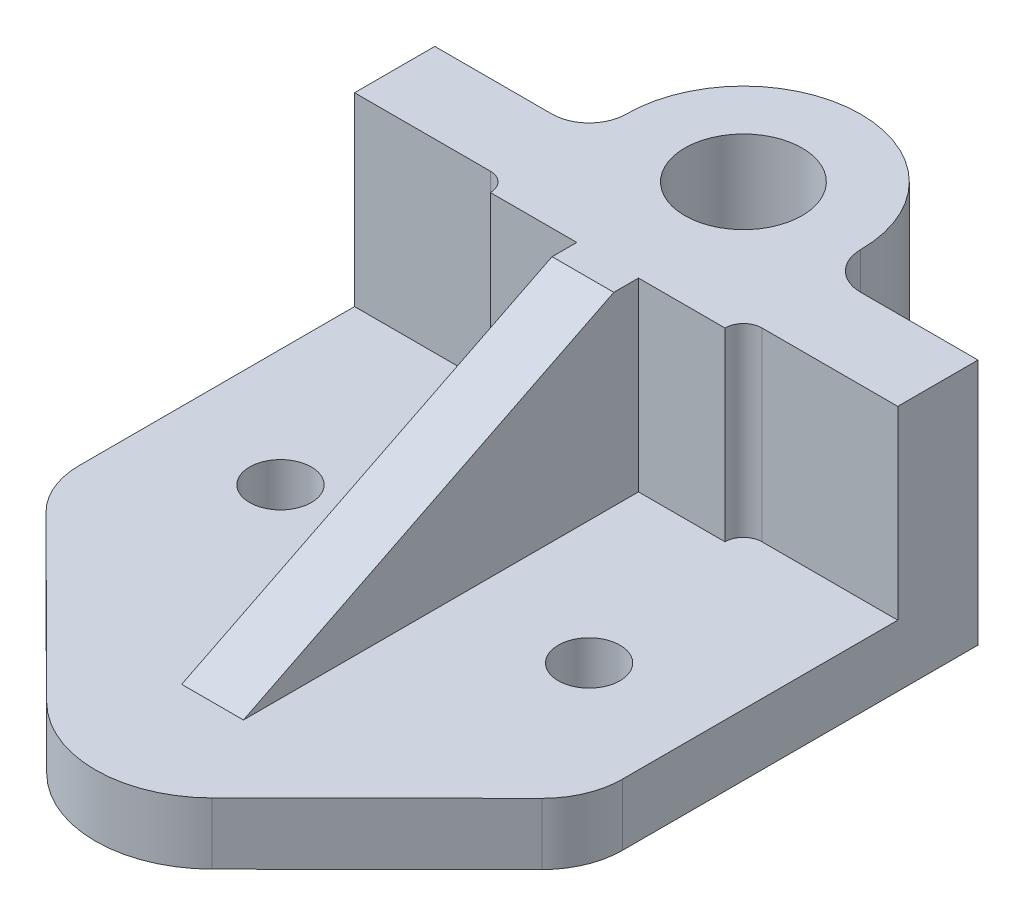
ISO-10303-21;
HEADER;
FILE_DESCRIPTION(('STEP AP214'),'2;1');
FILE_NAME('part.step','',(''),(''),'','','');
FILE_SCHEMA(('AUTOMOTIVE_DESIGN { 1 0 10303 214 1 1 1 1 }'));
ENDSEC;
DATA;
#1=APPLICATION_CONTEXT('core data for automotive mechanical design processes');
#2=APPLICATION_PROTOCOL_DEFINITION('international standard','automotive_design',2000,#1);
#3=PRODUCT_CONTEXT('',#1,'mechanical');
#4=PRODUCT('Part','Part','',(#3));
#5=PRODUCT_RELATED_PRODUCT_CATEGORY('part','',(#4));
#6=PRODUCT_DEFINITION_FORMATION('','',#4);
#7=PRODUCT_DEFINITION_CONTEXT('part definition',#1,'design');
#8=PRODUCT_DEFINITION('design','',#6,#7);
#9=PRODUCT_DEFINITION_SHAPE('','',#8);
#10=(LENGTH_UNIT() NAMED_UNIT(*) SI_UNIT(.MILLI.,.METRE.));
#11=(NAMED_UNIT(*) PLANE_ANGLE_UNIT() SI_UNIT($,.RADIAN.));
#12=(NAMED_UNIT(*) SI_UNIT($,.STERADIAN.) SOLID_ANGLE_UNIT());
#13=UNCERTAINTY_MEASURE_WITH_UNIT(LENGTH_MEASURE(1.E-05),#10,'distance_accuracy_value','');
#14=(GEOMETRIC_REPRESENTATION_CONTEXT(3) GLOBAL_UNCERTAINTY_ASSIGNED_CONTEXT((#13)) GLOBAL_UNIT_ASSIGNED_CONTEXT((#10,
#11,#12)) REPRESENTATION_CONTEXT('',''));
#15=CARTESIAN_POINT('',(0.,0.,0.));
#16=DIRECTION('',(0.,0.,1.));
#17=DIRECTION('',(1.,0.,0.));
#18=AXIS2_PLACEMENT_3D('',#15,#16,#17);
#19=CARTESIAN_POINT('',(-44.,40.,-6.5));
#20=DIRECTION('',(0.,0.,1.));
#21=DIRECTION('',(1.,0.,0.));
#22=AXIS2_PLACEMENT_3D('',#19,#20,#21);
#23=PLANE('',#22);
#24=DIRECTION('',(-1.,0.,0.));
#25=VECTOR('',#24,1.);
#26=CARTESIAN_POINT('',(-44.,0.,-6.5));
#27=LINE('',#26,#25);
#28=CARTESIAN_POINT('',(44.,0.,-6.5));
#29=VERTEX_POINT('',#28);
#30=CARTESIAN_POINT('',(25.,0.,-6.5));
#31=VERTEX_POINT('',#30);
#32=EDGE_CURVE('E291',#29,#31,#27,.T.);
#33=ORIENTED_EDGE('',*,*,#32,.T.);
#34=DIRECTION('',(0.,1.,0.));
#35=VECTOR('',#34,1.);
#36=CARTESIAN_POINT('',(25.,40.,-6.5));
#37=LINE('',#36,#35);
#38=CARTESIAN_POINT('',(25.,40.,-6.5));
#39=VERTEX_POINT('',#38);
#40=EDGE_CURVE('E339',#31,#39,#37,.T.);
#41=ORIENTED_EDGE('',*,*,#40,.T.);
#42=DIRECTION('',(-1.,0.,0.));
#43=VECTOR('',#42,1.);
#44=CARTESIAN_POINT('',(-44.,40.,-6.5));
#45=LINE('',#44,#43);
#46=CARTESIAN_POINT('',(44.,40.,-6.5));
#47=VERTEX_POINT('',#46);
#48=EDGE_CURVE('E281',#47,#39,#45,.T.);
#49=ORIENTED_EDGE('',*,*,#48,.F.);
#50=DIRECTION('',(0.,-1.,0.));
#51=VECTOR('',#50,1.);
#52=CARTESIAN_POINT('',(44.,40.,-6.5));
#53=LINE('',#52,#51);
#54=EDGE_CURVE('E306',#47,#29,#53,.T.);
#55=ORIENTED_EDGE('',*,*,#54,.T.);
#56=EDGE_LOOP('',(#33,#41,#49,#55));
#57=FACE_BOUND('',#56,.T.);
#58=ADVANCED_FACE('F44',(#57),#23,.F.);
#59=CARTESIAN_POINT('',(-44.,10.,56.5));
#60=DIRECTION('',(0.,-1.,0.));
#61=DIRECTION('',(1.,0.,0.));
#62=AXIS2_PLACEMENT_3D('',#59,#60,#61);
#63=PLANE('',#62);
#64=CARTESIAN_POINT('',(-25.,10.,37.5));
#65=DIRECTION('',(0.,1.,0.));
#66=DIRECTION('',(-1.,0.,0.));
#67=AXIS2_PLACEMENT_3D('',#64,#65,#66);
#68=CIRCLE('',#67,5.);
#69=CARTESIAN_POINT('',(-30.,10.,37.5));
#70=VERTEX_POINT('',#69);
#71=EDGE_CURVE('E382',#70,#70,#68,.T.);
#72=ORIENTED_EDGE('',*,*,#71,.F.);
#73=EDGE_LOOP('',(#72));
#74=FACE_BOUND('',#73,.T.);
#75=CARTESIAN_POINT('',(25.,10.,37.5));
#76=DIRECTION('',(0.,1.,0.));
#77=DIRECTION('',(-1.,0.,0.));
#78=AXIS2_PLACEMENT_3D('',#75,#76,#77);
#79=CIRCLE('',#78,5.);
#80=CARTESIAN_POINT('',(20.,10.,37.5));
#81=VERTEX_POINT('',#80);
#82=EDGE_CURVE('E222',#81,#81,#79,.T.);
#83=ORIENTED_EDGE('',*,*,#82,.F.);
#84=EDGE_LOOP('',(#83));
#85=FACE_BOUND('',#84,.T.);
#86=DIRECTION('',(0.,0.,-1.));
#87=VECTOR('',#86,1.);
#88=CARTESIAN_POINT('',(5.,10.,13.5));
#89=LINE('',#88,#87);
#90=CARTESIAN_POINT('',(5.,10.,73.5));
#91=VERTEX_POINT('',#90);
#92=CARTESIAN_POINT('',(5.,10.,9.5));
#93=VERTEX_POINT('',#92);
#94=EDGE_CURVE('E201',#91,#93,#89,.T.);
#95=ORIENTED_EDGE('',*,*,#94,.F.);
#96=DIRECTION('',(-1.,0.,0.));
#97=VECTOR('',#96,1.);
#98=CARTESIAN_POINT('',(-44.,10.,73.5));
#99=LINE('',#98,#97);
#100=CARTESIAN_POINT('',(-5.,10.,73.5));
#101=VERTEX_POINT('',#100);
#102=EDGE_CURVE('E219',#91,#101,#99,.T.);
#103=ORIENTED_EDGE('',*,*,#102,.T.);
#104=DIRECTION('',(0.,0.,-1.));
#105=VECTOR('',#104,1.);
#106=CARTESIAN_POINT('',(-5.,10.,13.5));
#107=LINE('',#106,#105);
#108=CARTESIAN_POINT('',(-5.,10.,9.5));
#109=VERTEX_POINT('',#108);
#110=EDGE_CURVE('E235',#101,#109,#107,.T.);
#111=ORIENTED_EDGE('',*,*,#110,.T.);
#112=DIRECTION('',(1.,0.,0.));
#113=VECTOR('',#112,1.);
#114=CARTESIAN_POINT('',(-19.,10.,9.5));
#115=LINE('',#114,#113);
#116=CARTESIAN_POINT('',(-19.,10.,9.5));
#117=VERTEX_POINT('',#116);
#118=EDGE_CURVE('E238',#117,#109,#115,.T.);
#119=ORIENTED_EDGE('',*,*,#118,.F.);
#120=CARTESIAN_POINT('',(-22.,10.,9.5));
#121=DIRECTION('',(0.,-1.,0.));
#122=DIRECTION('',(1.,0.,0.));
#123=AXIS2_PLACEMENT_3D('',#120,#121,#122);
#124=CIRCLE('',#123,3.);
#125=CARTESIAN_POINT('',(-22.,10.,6.5));
#126=VERTEX_POINT('',#125);
#127=EDGE_CURVE('E328',#117,#126,#124,.F.);
#128=ORIENTED_EDGE('',*,*,#127,.T.);
#129=DIRECTION('',(-1.,0.,0.));
#130=VECTOR('',#129,1.);
#131=CARTESIAN_POINT('',(-44.,10.,6.5));
#132=LINE('',#131,#130);
#133=CARTESIAN_POINT('',(-44.,10.,6.5));
#134=VERTEX_POINT('',#133);
#135=EDGE_CURVE('E262',#126,#134,#132,.T.);
#136=ORIENTED_EDGE('',*,*,#135,.T.);
#137=DIRECTION('',(0.,0.,-1.));
#138=VECTOR('',#137,1.);
#139=CARTESIAN_POINT('',(-44.,10.,56.5));
#140=LINE('',#139,#138);
#141=CARTESIAN_POINT('',(-44.,10.,51.0990021941588));
#142=VERTEX_POINT('',#141);
#143=EDGE_CURVE('E272',#142,#134,#140,.T.);
#144=ORIENTED_EDGE('',*,*,#143,.F.);
#145=CARTESIAN_POINT('',(-31.,10.,51.0990021941588));
#146=DIRECTION('',(0.,-1.,0.));
#147=DIRECTION('',(1.,0.,0.));
#148=AXIS2_PLACEMENT_3D('',#145,#146,#147);
#149=CIRCLE('',#148,13.);
#150=CARTESIAN_POINT('',(-40.1727948989015,10.,60.3109419324922));
#151=VERTEX_POINT('',#150);
#152=EDGE_CURVE('E315',#142,#151,#149,.F.);
#153=ORIENTED_EDGE('',*,*,#152,.T.);
#154=DIRECTION('',(0.708610749102569,0.,0.705599607607811));
#155=VECTOR('',#154,1.);
#156=CARTESIAN_POINT('',(-44.,10.,56.5));
#157=LINE('',#156,#155);
#158=CARTESIAN_POINT('',(-13.4063925445484,10.,86.9636042329488));
#159=VERTEX_POINT('',#158);
#160=EDGE_CURVE('E250',#151,#159,#157,.T.);
#161=ORIENTED_EDGE('',*,*,#160,.T.);
#162=CARTESIAN_POINT('',(0.,10.,73.5));
#163=DIRECTION('',(0.,1.,0.));
#164=DIRECTION('',(-1.,0.,0.));
#165=AXIS2_PLACEMENT_3D('',#162,#163,#164);
#166=CIRCLE('',#165,19.);
#167=CARTESIAN_POINT('',(13.4063925445484,10.,86.9636042329488));
#168=VERTEX_POINT('',#167);
#169=EDGE_CURVE('E259',#159,#168,#166,.T.);
#170=ORIENTED_EDGE('',*,*,#169,.T.);
#171=DIRECTION('',(0.708610749102569,0.,-0.705599607607811));
#172=VECTOR('',#171,1.);
#173=CARTESIAN_POINT('',(44.,10.,56.5));
#174=LINE('',#173,#172);
#175=CARTESIAN_POINT('',(40.1727948989016,10.,60.3109419324922));
#176=VERTEX_POINT('',#175);
#177=EDGE_CURVE('E252',#168,#176,#174,.T.);
#178=ORIENTED_EDGE('',*,*,#177,.T.);
#179=CARTESIAN_POINT('',(31.,10.,51.0990021941588));
#180=DIRECTION('',(0.,-1.,0.));
#181=DIRECTION('',(1.,0.,0.));
#182=AXIS2_PLACEMENT_3D('',#179,#180,#181);
#183=CIRCLE('',#182,13.);
#184=CARTESIAN_POINT('',(44.,10.,51.0990021941588));
#185=VERTEX_POINT('',#184);
#186=EDGE_CURVE('E313',#176,#185,#183,.F.);
#187=ORIENTED_EDGE('',*,*,#186,.T.);
#188=DIRECTION('',(0.,0.,-1.));
#189=VECTOR('',#188,1.);
#190=CARTESIAN_POINT('',(44.,10.,56.5));
#191=LINE('',#190,#189);
#192=CARTESIAN_POINT('',(44.,10.,6.5));
#193=VERTEX_POINT('',#192);
#194=EDGE_CURVE('E274',#185,#193,#191,.T.);
#195=ORIENTED_EDGE('',*,*,#194,.T.);
#196=CARTESIAN_POINT('',(22.,10.,6.5));
#197=VERTEX_POINT('',#196);
#198=EDGE_CURVE('E268',#193,#197,#132,.T.);
#199=ORIENTED_EDGE('',*,*,#198,.T.);
#200=CARTESIAN_POINT('',(22.,10.,9.5));
#201=DIRECTION('',(0.,-1.,0.));
#202=DIRECTION('',(1.,0.,0.));
#203=AXIS2_PLACEMENT_3D('',#200,#201,#202);
#204=CIRCLE('',#203,3.);
#205=CARTESIAN_POINT('',(19.,10.,9.5));
#206=VERTEX_POINT('',#205);
#207=EDGE_CURVE('E331',#197,#206,#204,.F.);
#208=ORIENTED_EDGE('',*,*,#207,.T.);
#209=EDGE_CURVE('E240',#93,#206,#115,.T.);
#210=ORIENTED_EDGE('',*,*,#209,.F.);
#211=EDGE_LOOP('',(#95,#103,#111,#119,#128,#136,#144,#153,#161,#170,#178,#187,#195,#199,#208,#210));
#212=FACE_BOUND('',#211,.T.);
#213=ADVANCED_FACE('F391',(#74,#85,#212),#63,.F.);
#214=CARTESIAN_POINT('',(0.,0.,9.5));
#215=DIRECTION('',(0.,0.,1.));
#216=DIRECTION('',(1.,0.,0.));
#217=AXIS2_PLACEMENT_3D('',#214,#215,#216);
#218=PLANE('',#217);
#219=ORIENTED_EDGE('',*,*,#118,.T.);
#220=DIRECTION('',(0.,-1.,0.));
#221=VECTOR('',#220,1.);
#222=CARTESIAN_POINT('',(-5.,40.,9.5));
#223=LINE('',#222,#221);
#224=CARTESIAN_POINT('',(-5.,40.,9.5));
#225=VERTEX_POINT('',#224);
#226=EDGE_CURVE('E218',#225,#109,#223,.T.);
#227=ORIENTED_EDGE('',*,*,#226,.F.);
#228=DIRECTION('',(-1.,0.,0.));
#229=VECTOR('',#228,1.);
#230=CARTESIAN_POINT('',(-19.,40.,9.5));
#231=LINE('',#230,#229);
#232=CARTESIAN_POINT('',(-19.,40.,9.5));
#233=VERTEX_POINT('',#232);
#234=EDGE_CURVE('E242',#225,#233,#231,.T.);
#235=ORIENTED_EDGE('',*,*,#234,.T.);
#236=DIRECTION('',(0.,-1.,0.));
#237=VECTOR('',#236,1.);
#238=CARTESIAN_POINT('',(-19.,40.,9.5));
#239=LINE('',#238,#237);
#240=EDGE_CURVE('E234',#233,#117,#239,.T.);
#241=ORIENTED_EDGE('',*,*,#240,.T.);
#242=EDGE_LOOP('',(#219,#227,#235,#241));
#243=FACE_BOUND('',#242,.T.);
#244=ADVANCED_FACE('F392',(#243),#218,.T.);
#245=CARTESIAN_POINT('',(19.,40.,9.5));
#246=VERTEX_POINT('',#245);
#247=CARTESIAN_POINT('',(4.99999999999999,40.,9.5));
#248=VERTEX_POINT('',#247);
#249=EDGE_CURVE('E244',#246,#248,#231,.T.);
#250=ORIENTED_EDGE('',*,*,#249,.T.);
#251=DIRECTION('',(0.,1.,0.));
#252=VECTOR('',#251,1.);
#253=CARTESIAN_POINT('',(5.,40.,9.5));
#254=LINE('',#253,#252);
#255=EDGE_CURVE('E198',#93,#248,#254,.T.);
#256=ORIENTED_EDGE('',*,*,#255,.F.);
#257=ORIENTED_EDGE('',*,*,#209,.T.);
#258=DIRECTION('',(0.,1.,0.));
#259=VECTOR('',#258,1.);
#260=CARTESIAN_POINT('',(19.,40.,9.5));
#261=LINE('',#260,#259);
#262=EDGE_CURVE('E241',#206,#246,#261,.T.);
#263=ORIENTED_EDGE('',*,*,#262,.T.);
#264=EDGE_LOOP('',(#250,#256,#257,#263));
#265=FACE_BOUND('',#264,.T.);
#266=ADVANCED_FACE('F401',(#265),#218,.T.);
#267=CARTESIAN_POINT('',(-44.,40.,6.5));
#268=DIRECTION('',(0.,0.,-1.));
#269=DIRECTION('',(-1.,0.,0.));
#270=AXIS2_PLACEMENT_3D('',#267,#268,#269);
#271=PLANE('',#270);
#272=ORIENTED_EDGE('',*,*,#135,.F.);
#273=DIRECTION('',(0.,-1.,0.));
#274=VECTOR('',#273,1.);
#275=CARTESIAN_POINT('',(-22.,40.,6.5));
#276=LINE('',#275,#274);
#277=CARTESIAN_POINT('',(-22.,40.,6.5));
#278=VERTEX_POINT('',#277);
#279=EDGE_CURVE('E333',#126,#278,#276,.F.);
#280=ORIENTED_EDGE('',*,*,#279,.T.);
#281=DIRECTION('',(1.,0.,0.));
#282=VECTOR('',#281,1.);
#283=CARTESIAN_POINT('',(-44.,40.,6.5));
#284=LINE('',#283,#282);
#285=CARTESIAN_POINT('',(-44.,40.,6.5));
#286=VERTEX_POINT('',#285);
#287=EDGE_CURVE('E290',#286,#278,#284,.T.);
#288=ORIENTED_EDGE('',*,*,#287,.F.);
#289=DIRECTION('',(0.,-1.,0.));
#290=VECTOR('',#289,1.);
#291=CARTESIAN_POINT('',(-44.,40.,6.5));
#292=LINE('',#291,#290);
#293=EDGE_CURVE('E297',#286,#134,#292,.T.);
#294=ORIENTED_EDGE('',*,*,#293,.T.);
#295=EDGE_LOOP('',(#272,#280,#288,#294));
#296=FACE_BOUND('',#295,.T.);
#297=ADVANCED_FACE('F449',(#296),#271,.F.);
#298=CARTESIAN_POINT('',(22.,40.,6.5));
#299=VERTEX_POINT('',#298);
#300=CARTESIAN_POINT('',(44.,40.,6.5));
#301=VERTEX_POINT('',#300);
#302=EDGE_CURVE('E286',#299,#301,#284,.T.);
#303=ORIENTED_EDGE('',*,*,#302,.F.);
#304=DIRECTION('',(0.,1.,0.));
#305=VECTOR('',#304,1.);
#306=CARTESIAN_POINT('',(22.,10.,6.5));
#307=LINE('',#306,#305);
#308=EDGE_CURVE('E326',#299,#197,#307,.F.);
#309=ORIENTED_EDGE('',*,*,#308,.T.);
#310=ORIENTED_EDGE('',*,*,#198,.F.);
#311=DIRECTION('',(0.,-1.,0.));
#312=VECTOR('',#311,1.);
#313=CARTESIAN_POINT('',(44.,40.,6.5));
#314=LINE('',#313,#312);
#315=EDGE_CURVE('E289',#301,#193,#314,.T.);
#316=ORIENTED_EDGE('',*,*,#315,.F.);
#317=EDGE_LOOP('',(#303,#309,#310,#316));
#318=FACE_BOUND('',#317,.T.);
#319=ADVANCED_FACE('F408',(#318),#271,.F.);
#320=CARTESIAN_POINT('',(44.,40.,6.5));
#321=DIRECTION('',(-1.,0.,0.));
#322=DIRECTION('',(0.,0.,1.));
#323=AXIS2_PLACEMENT_3D('',#320,#321,#322);
#324=PLANE('',#323);
#325=ORIENTED_EDGE('',*,*,#194,.F.);
#326=DIRECTION('',(0.,1.,0.));
#327=VECTOR('',#326,1.);
#328=CARTESIAN_POINT('',(44.,0.,51.0990021941588));
#329=LINE('',#328,#327);
#330=CARTESIAN_POINT('',(44.,0.,51.0990021941588));
#331=VERTEX_POINT('',#330);
#332=EDGE_CURVE('E317',#185,#331,#329,.F.);
#333=ORIENTED_EDGE('',*,*,#332,.T.);
#334=DIRECTION('',(0.,0.,-1.));
#335=VECTOR('',#334,1.);
#336=CARTESIAN_POINT('',(44.,0.,6.5));
#337=LINE('',#336,#335);
#338=EDGE_CURVE('E277',#331,#29,#337,.T.);
#339=ORIENTED_EDGE('',*,*,#338,.T.);
#340=ORIENTED_EDGE('',*,*,#54,.F.);
#341=DIRECTION('',(0.,0.,-1.));
#342=VECTOR('',#341,1.);
#343=CARTESIAN_POINT('',(44.,40.,6.5));
#344=LINE('',#343,#342);
#345=EDGE_CURVE('E280',#301,#47,#344,.T.);
#346=ORIENTED_EDGE('',*,*,#345,.F.);
#347=ORIENTED_EDGE('',*,*,#315,.T.);
#348=EDGE_LOOP('',(#325,#333,#339,#340,#346,#347));
#349=FACE_BOUND('',#348,.T.);
#350=ADVANCED_FACE('F412',(#349),#324,.F.);
#351=CARTESIAN_POINT('',(-25.,40.,-6.5));
#352=VERTEX_POINT('',#351);
#353=CARTESIAN_POINT('',(-44.,40.,-6.5));
#354=VERTEX_POINT('',#353);
#355=EDGE_CURVE('E278',#352,#354,#45,.T.);
#356=ORIENTED_EDGE('',*,*,#355,.F.);
#357=DIRECTION('',(0.,1.,0.));
#358=VECTOR('',#357,1.);
#359=CARTESIAN_POINT('',(-25.,40.,-6.5));
#360=LINE('',#359,#358);
#361=CARTESIAN_POINT('',(-25.,0.,-6.5));
#362=VERTEX_POINT('',#361);
#363=EDGE_CURVE('E58',#352,#362,#360,.F.);
#364=ORIENTED_EDGE('',*,*,#363,.T.);
#365=CARTESIAN_POINT('',(-44.,0.,-6.5));
#366=VERTEX_POINT('',#365);
#367=EDGE_CURVE('E292',#362,#366,#27,.T.);
#368=ORIENTED_EDGE('',*,*,#367,.T.);
#369=DIRECTION('',(0.,-1.,0.));
#370=VECTOR('',#369,1.);
#371=CARTESIAN_POINT('',(-44.,40.,-6.5));
#372=LINE('',#371,#370);
#373=EDGE_CURVE('E303',#354,#366,#372,.T.);
#374=ORIENTED_EDGE('',*,*,#373,.F.);
#375=EDGE_LOOP('',(#356,#364,#368,#374));
#376=FACE_BOUND('',#375,.T.);
#377=ADVANCED_FACE('F472',(#376),#23,.F.);
#378=CARTESIAN_POINT('',(-44.,40.,6.5));
#379=DIRECTION('',(1.,0.,0.));
#380=DIRECTION('',(0.,0.,-1.));
#381=AXIS2_PLACEMENT_3D('',#378,#379,#380);
#382=PLANE('',#381);
#383=DIRECTION('',(0.,0.,1.));
#384=VECTOR('',#383,1.);
#385=CARTESIAN_POINT('',(-44.,0.,6.5));
#386=LINE('',#385,#384);
#387=CARTESIAN_POINT('',(-44.,0.,51.0990021941588));
#388=VERTEX_POINT('',#387);
#389=EDGE_CURVE('E284',#366,#388,#386,.T.);
#390=ORIENTED_EDGE('',*,*,#389,.T.);
#391=DIRECTION('',(0.,-1.,0.));
#392=VECTOR('',#391,1.);
#393=CARTESIAN_POINT('',(-44.,10.,51.0990021941588));
#394=LINE('',#393,#392);
#395=EDGE_CURVE('E323',#388,#142,#394,.F.);
#396=ORIENTED_EDGE('',*,*,#395,.T.);
#397=ORIENTED_EDGE('',*,*,#143,.T.);
#398=ORIENTED_EDGE('',*,*,#293,.F.);
#399=DIRECTION('',(0.,0.,1.));
#400=VECTOR('',#399,1.);
#401=CARTESIAN_POINT('',(-44.,40.,6.5));
#402=LINE('',#401,#400);
#403=EDGE_CURVE('E283',#354,#286,#402,.T.);
#404=ORIENTED_EDGE('',*,*,#403,.F.);
#405=ORIENTED_EDGE('',*,*,#373,.T.);
#406=EDGE_LOOP('',(#390,#396,#397,#398,#404,#405));
#407=FACE_BOUND('',#406,.T.);
#408=ADVANCED_FACE('F445',(#407),#382,.F.);
#409=CARTESIAN_POINT('',(0.,40.,0.));
#410=DIRECTION('',(0.,-1.,0.));
#411=DIRECTION('',(0.,0.,-1.));
#412=AXIS2_PLACEMENT_3D('',#409,#410,#411);
#413=PLANE('',#412);
#414=CARTESIAN_POINT('',(0.,40.,-12.5));
#415=DIRECTION('',(0.,1.,0.));
#416=DIRECTION('',(0.,0.,1.));
#417=AXIS2_PLACEMENT_3D('',#414,#415,#416);
#418=CIRCLE('',#417,9.5);
#419=CARTESIAN_POINT('',(0.,40.,-3.));
#420=VERTEX_POINT('',#419);
#421=EDGE_CURVE('E374',#420,#420,#418,.T.);
#422=ORIENTED_EDGE('',*,*,#421,.F.);
#423=EDGE_LOOP('',(#422));
#424=FACE_BOUND('',#423,.T.);
#425=ORIENTED_EDGE('',*,*,#48,.T.);
#426=CARTESIAN_POINT('',(25.,40.,-12.5));
#427=DIRECTION('',(0.,-1.,0.));
#428=DIRECTION('',(0.,0.,-1.));
#429=AXIS2_PLACEMENT_3D('',#426,#427,#428);
#430=CIRCLE('',#429,6.);
#431=CARTESIAN_POINT('',(19.,40.,-12.5));
#432=VERTEX_POINT('',#431);
#433=EDGE_CURVE('E350',#39,#432,#430,.T.);
#434=ORIENTED_EDGE('',*,*,#433,.T.);
#435=CARTESIAN_POINT('',(0.,40.,-12.5));
#436=DIRECTION('',(0.,1.,0.));
#437=DIRECTION('',(0.,0.,1.));
#438=AXIS2_PLACEMENT_3D('',#435,#436,#437);
#439=CIRCLE('',#438,19.);
#440=CARTESIAN_POINT('',(-19.,40.,-12.5));
#441=VERTEX_POINT('',#440);
#442=EDGE_CURVE('E370',#432,#441,#439,.T.);
#443=ORIENTED_EDGE('',*,*,#442,.T.);
#444=CARTESIAN_POINT('',(-25.,40.,-12.5));
#445=DIRECTION('',(0.,-1.,0.));
#446=DIRECTION('',(0.,0.,-1.));
#447=AXIS2_PLACEMENT_3D('',#444,#445,#446);
#448=CIRCLE('',#447,6.);
#449=EDGE_CURVE('E52',#441,#352,#448,.T.);
#450=ORIENTED_EDGE('',*,*,#449,.T.);
#451=ORIENTED_EDGE('',*,*,#355,.T.);
#452=ORIENTED_EDGE('',*,*,#403,.T.);
#453=ORIENTED_EDGE('',*,*,#287,.T.);
#454=CARTESIAN_POINT('',(-22.,40.,9.5));
#455=DIRECTION('',(0.,-1.,0.));
#456=DIRECTION('',(0.,0.,-1.));
#457=AXIS2_PLACEMENT_3D('',#454,#455,#456);
#458=CIRCLE('',#457,3.);
#459=EDGE_CURVE('E340',#278,#233,#458,.T.);
#460=ORIENTED_EDGE('',*,*,#459,.T.);
#461=ORIENTED_EDGE('',*,*,#234,.F.);
#462=DIRECTION('',(0.,0.,-1.));
#463=VECTOR('',#462,1.);
#464=CARTESIAN_POINT('',(-5.,40.,13.5));
#465=LINE('',#464,#463);
#466=CARTESIAN_POINT('',(-5.,40.,13.5));
#467=VERTEX_POINT('',#466);
#468=EDGE_CURVE('E205',#467,#225,#465,.T.);
#469=ORIENTED_EDGE('',*,*,#468,.F.);
#470=DIRECTION('',(-1.,0.,0.));
#471=VECTOR('',#470,1.);
#472=CARTESIAN_POINT('',(-5.,40.,13.5));
#473=LINE('',#472,#471);
#474=CARTESIAN_POINT('',(5.,40.,13.5));
#475=VERTEX_POINT('',#474);
#476=EDGE_CURVE('E204',#475,#467,#473,.T.);
#477=ORIENTED_EDGE('',*,*,#476,.F.);
#478=DIRECTION('',(0.,0.,-1.));
#479=VECTOR('',#478,1.);
#480=CARTESIAN_POINT('',(5.,40.,13.5));
#481=LINE('',#480,#479);
#482=EDGE_CURVE('E194',#475,#248,#481,.T.);
#483=ORIENTED_EDGE('',*,*,#482,.T.);
#484=ORIENTED_EDGE('',*,*,#249,.F.);
#485=CARTESIAN_POINT('',(22.,40.,9.5));
#486=DIRECTION('',(0.,-1.,0.));
#487=DIRECTION('',(0.,0.,-1.));
#488=AXIS2_PLACEMENT_3D('',#485,#486,#487);
#489=CIRCLE('',#488,3.);
#490=EDGE_CURVE('E334',#246,#299,#489,.T.);
#491=ORIENTED_EDGE('',*,*,#490,.T.);
#492=ORIENTED_EDGE('',*,*,#302,.T.);
#493=ORIENTED_EDGE('',*,*,#345,.T.);
#494=EDGE_LOOP('',(#425,#434,#443,#450,#451,#452,#453,#460,#461,#469,#477,#483,#484,#491,#492,#493));
#495=FACE_BOUND('',#494,.T.);
#496=ADVANCED_FACE('F210',(#424,#495),#413,.F.);
#497=CARTESIAN_POINT('',(0.,0.,0.));
#498=DIRECTION('',(0.,-1.,0.));
#499=DIRECTION('',(0.,0.,-1.));
#500=AXIS2_PLACEMENT_3D('',#497,#498,#499);
#501=PLANE('',#500);
#502=CARTESIAN_POINT('',(0.,0.,-12.5));
#503=DIRECTION('',(0.,1.,0.));
#504=DIRECTION('',(0.,0.,1.));
#505=AXIS2_PLACEMENT_3D('',#502,#503,#504);
#506=CIRCLE('',#505,9.5);
#507=CARTESIAN_POINT('',(0.,0.,-3.));
#508=VERTEX_POINT('',#507);
#509=EDGE_CURVE('E371',#508,#508,#506,.T.);
#510=ORIENTED_EDGE('',*,*,#509,.T.);
#511=EDGE_LOOP('',(#510));
#512=FACE_BOUND('',#511,.T.);
#513=CARTESIAN_POINT('',(-25.,0.,37.5));
#514=DIRECTION('',(0.,1.,0.));
#515=DIRECTION('',(-1.,0.,0.));
#516=AXIS2_PLACEMENT_3D('',#513,#514,#515);
#517=CIRCLE('',#516,5.);
#518=CARTESIAN_POINT('',(-30.,0.,37.5));
#519=VERTEX_POINT('',#518);
#520=EDGE_CURVE('E221',#519,#519,#517,.T.);
#521=ORIENTED_EDGE('',*,*,#520,.T.);
#522=EDGE_LOOP('',(#521));
#523=FACE_BOUND('',#522,.T.);
#524=CARTESIAN_POINT('',(25.,0.,37.5));
#525=DIRECTION('',(0.,1.,0.));
#526=DIRECTION('',(-1.,0.,0.));
#527=AXIS2_PLACEMENT_3D('',#524,#525,#526);
#528=CIRCLE('',#527,5.);
#529=CARTESIAN_POINT('',(20.,0.,37.5));
#530=VERTEX_POINT('',#529);
#531=EDGE_CURVE('E384',#530,#530,#528,.T.);
#532=ORIENTED_EDGE('',*,*,#531,.T.);
#533=EDGE_LOOP('',(#532));
#534=FACE_BOUND('',#533,.T.);
#535=DIRECTION('',(0.708610749102569,0.,-0.705599607607811));
#536=VECTOR('',#535,1.);
#537=CARTESIAN_POINT('',(44.,0.,56.5));
#538=LINE('',#537,#536);
#539=CARTESIAN_POINT('',(13.4063925445484,0.,86.9636042329488));
#540=VERTEX_POINT('',#539);
#541=CARTESIAN_POINT('',(40.1727948989016,0.,60.3109419324922));
#542=VERTEX_POINT('',#541);
#543=EDGE_CURVE('E254',#540,#542,#538,.T.);
#544=ORIENTED_EDGE('',*,*,#543,.F.);
#545=CARTESIAN_POINT('',(0.,0.,73.5));
#546=DIRECTION('',(0.,1.,0.));
#547=DIRECTION('',(-1.,0.,0.));
#548=AXIS2_PLACEMENT_3D('',#545,#546,#547);
#549=CIRCLE('',#548,19.);
#550=CARTESIAN_POINT('',(-13.4063925445484,0.,86.9636042329488));
#551=VERTEX_POINT('',#550);
#552=EDGE_CURVE('E249',#551,#540,#549,.T.);
#553=ORIENTED_EDGE('',*,*,#552,.F.);
#554=DIRECTION('',(0.708610749102569,0.,0.705599607607811));
#555=VECTOR('',#554,1.);
#556=CARTESIAN_POINT('',(-44.,0.,56.5));
#557=LINE('',#556,#555);
#558=CARTESIAN_POINT('',(-40.1727948989015,0.,60.3109419324922));
#559=VERTEX_POINT('',#558);
#560=EDGE_CURVE('E247',#559,#551,#557,.T.);
#561=ORIENTED_EDGE('',*,*,#560,.F.);
#562=CARTESIAN_POINT('',(-31.,0.,51.0990021941588));
#563=DIRECTION('',(0.,-1.,0.));
#564=DIRECTION('',(0.,0.,-1.));
#565=AXIS2_PLACEMENT_3D('',#562,#563,#564);
#566=CIRCLE('',#565,13.);
#567=EDGE_CURVE('E319',#559,#388,#566,.T.);
#568=ORIENTED_EDGE('',*,*,#567,.T.);
#569=ORIENTED_EDGE('',*,*,#389,.F.);
#570=ORIENTED_EDGE('',*,*,#367,.F.);
#571=CARTESIAN_POINT('',(-25.,0.,-12.5));
#572=DIRECTION('',(0.,-1.,0.));
#573=DIRECTION('',(0.,0.,-1.));
#574=AXIS2_PLACEMENT_3D('',#571,#572,#573);
#575=CIRCLE('',#574,6.);
#576=CARTESIAN_POINT('',(-19.,0.,-12.5));
#577=VERTEX_POINT('',#576);
#578=EDGE_CURVE('E11',#362,#577,#575,.F.);
#579=ORIENTED_EDGE('',*,*,#578,.T.);
#580=CARTESIAN_POINT('',(0.,0.,-12.5));
#581=DIRECTION('',(0.,1.,0.));
#582=DIRECTION('',(0.,0.,1.));
#583=AXIS2_PLACEMENT_3D('',#580,#581,#582);
#584=CIRCLE('',#583,19.);
#585=CARTESIAN_POINT('',(19.,0.,-12.5));
#586=VERTEX_POINT('',#585);
#587=EDGE_CURVE('E360',#586,#577,#584,.T.);
#588=ORIENTED_EDGE('',*,*,#587,.F.);
#589=CARTESIAN_POINT('',(25.,0.,-12.5));
#590=DIRECTION('',(0.,-1.,0.));
#591=DIRECTION('',(0.,0.,-1.));
#592=AXIS2_PLACEMENT_3D('',#589,#590,#591);
#593=CIRCLE('',#592,6.);
#594=EDGE_CURVE('E347',#586,#31,#593,.F.);
#595=ORIENTED_EDGE('',*,*,#594,.T.);
#596=ORIENTED_EDGE('',*,*,#32,.F.);
#597=ORIENTED_EDGE('',*,*,#338,.F.);
#598=CARTESIAN_POINT('',(31.,0.,51.0990021941588));
#599=DIRECTION('',(0.,-1.,0.));
#600=DIRECTION('',(0.,0.,-1.));
#601=AXIS2_PLACEMENT_3D('',#598,#599,#600);
#602=CIRCLE('',#601,13.);
#603=EDGE_CURVE('E318',#331,#542,#602,.T.);
#604=ORIENTED_EDGE('',*,*,#603,.T.);
#605=EDGE_LOOP('',(#544,#553,#561,#568,#569,#570,#579,#588,#595,#596,#597,#604));
#606=FACE_BOUND('',#605,.T.);
#607=ADVANCED_FACE('F358',(#512,#523,#534,#606),#501,.T.);
#608=CARTESIAN_POINT('',(44.,0.,56.5));
#609=DIRECTION('',(0.705599607607811,0.,0.708610749102569));
#610=DIRECTION('',(0.708610749102569,0.,-0.705599607607811));
#611=AXIS2_PLACEMENT_3D('',#608,#609,#610);
#612=PLANE('',#611);
#613=ORIENTED_EDGE('',*,*,#543,.T.);
#614=DIRECTION('',(0.,1.,0.));
#615=VECTOR('',#614,1.);
#616=CARTESIAN_POINT('',(40.1727948989016,10.,60.3109419324922));
#617=LINE('',#616,#615);
#618=EDGE_CURVE('E307',#542,#176,#617,.T.);
#619=ORIENTED_EDGE('',*,*,#618,.T.);
#620=ORIENTED_EDGE('',*,*,#177,.F.);
#621=DIRECTION('',(0.,1.,0.));
#622=VECTOR('',#621,1.);
#623=CARTESIAN_POINT('',(13.4063925445484,0.,86.9636042329488));
#624=LINE('',#623,#622);
#625=EDGE_CURVE('E265',#540,#168,#624,.T.);
#626=ORIENTED_EDGE('',*,*,#625,.F.);
#627=EDGE_LOOP('',(#613,#619,#620,#626));
#628=FACE_BOUND('',#627,.T.);
#629=ADVANCED_FACE('F421',(#628),#612,.T.);
#630=CARTESIAN_POINT('',(0.,0.,73.5));
#631=DIRECTION('',(0.,1.,0.));
#632=DIRECTION('',(-1.,0.,0.));
#633=AXIS2_PLACEMENT_3D('',#630,#631,#632);
#634=CYLINDRICAL_SURFACE('',#633,19.);
#635=ORIENTED_EDGE('',*,*,#552,.T.);
#636=ORIENTED_EDGE('',*,*,#625,.T.);
#637=ORIENTED_EDGE('',*,*,#169,.F.);
#638=DIRECTION('',(0.,1.,0.));
#639=VECTOR('',#638,1.);
#640=CARTESIAN_POINT('',(-13.4063925445484,0.,86.9636042329488));
#641=LINE('',#640,#639);
#642=EDGE_CURVE('E257',#551,#159,#641,.T.);
#643=ORIENTED_EDGE('',*,*,#642,.F.);
#644=EDGE_LOOP('',(#635,#636,#637,#643));
#645=FACE_BOUND('',#644,.T.);
#646=ADVANCED_FACE('F429',(#645),#634,.T.);
#647=CARTESIAN_POINT('',(-44.,0.,56.5));
#648=DIRECTION('',(-0.705599607607811,0.,0.708610749102569));
#649=DIRECTION('',(0.708610749102569,0.,0.705599607607811));
#650=AXIS2_PLACEMENT_3D('',#647,#648,#649);
#651=PLANE('',#650);
#652=ORIENTED_EDGE('',*,*,#160,.F.);
#653=DIRECTION('',(0.,-1.,0.));
#654=VECTOR('',#653,1.);
#655=CARTESIAN_POINT('',(-40.1727948989015,0.,60.3109419324922));
#656=LINE('',#655,#654);
#657=EDGE_CURVE('E325',#151,#559,#656,.T.);
#658=ORIENTED_EDGE('',*,*,#657,.T.);
#659=ORIENTED_EDGE('',*,*,#560,.T.);
#660=ORIENTED_EDGE('',*,*,#642,.T.);
#661=EDGE_LOOP('',(#652,#658,#659,#660));
#662=FACE_BOUND('',#661,.T.);
#663=ADVANCED_FACE('F432',(#662),#651,.T.);
#664=CARTESIAN_POINT('',(31.,0.,51.0990021941588));
#665=DIRECTION('',(0.,-1.,0.));
#666=DIRECTION('',(0.,0.,-1.));
#667=AXIS2_PLACEMENT_3D('',#664,#665,#666);
#668=CYLINDRICAL_SURFACE('',#667,13.);
#669=ORIENTED_EDGE('',*,*,#603,.F.);
#670=ORIENTED_EDGE('',*,*,#332,.F.);
#671=ORIENTED_EDGE('',*,*,#186,.F.);
#672=ORIENTED_EDGE('',*,*,#618,.F.);
#673=EDGE_LOOP('',(#669,#670,#671,#672));
#674=FACE_BOUND('',#673,.T.);
#675=ADVANCED_FACE('F419',(#674),#668,.T.);
#676=CARTESIAN_POINT('',(-31.,0.,51.0990021941588));
#677=DIRECTION('',(0.,1.,0.));
#678=DIRECTION('',(0.,0.,1.));
#679=AXIS2_PLACEMENT_3D('',#676,#677,#678);
#680=CYLINDRICAL_SURFACE('',#679,13.);
#681=ORIENTED_EDGE('',*,*,#152,.F.);
#682=ORIENTED_EDGE('',*,*,#395,.F.);
#683=ORIENTED_EDGE('',*,*,#567,.F.);
#684=ORIENTED_EDGE('',*,*,#657,.F.);
#685=EDGE_LOOP('',(#681,#682,#683,#684));
#686=FACE_BOUND('',#685,.T.);
#687=ADVANCED_FACE('F438',(#686),#680,.T.);
#688=CARTESIAN_POINT('',(-5.,40.,13.5));
#689=DIRECTION('',(1.,0.,0.));
#690=DIRECTION('',(0.,1.,0.));
#691=AXIS2_PLACEMENT_3D('',#688,#689,#690);
#692=PLANE('',#691);
#693=ORIENTED_EDGE('',*,*,#226,.T.);
#694=ORIENTED_EDGE('',*,*,#110,.F.);
#695=DIRECTION('',(0.,-0.447213595499958,0.894427190999916));
#696=VECTOR('',#695,1.);
#697=CARTESIAN_POINT('',(-5.,40.,13.5));
#698=LINE('',#697,#696);
#699=EDGE_CURVE('E216',#467,#101,#698,.T.);
#700=ORIENTED_EDGE('',*,*,#699,.F.);
#701=ORIENTED_EDGE('',*,*,#468,.T.);
#702=EDGE_LOOP('',(#693,#694,#700,#701));
#703=FACE_BOUND('',#702,.T.);
#704=ADVANCED_FACE('F460',(#703),#692,.F.);
#705=CARTESIAN_POINT('',(5.,40.,13.5));
#706=DIRECTION('',(-1.,0.,0.));
#707=DIRECTION('',(0.,-1.,0.));
#708=AXIS2_PLACEMENT_3D('',#705,#706,#707);
#709=PLANE('',#708);
#710=ORIENTED_EDGE('',*,*,#255,.T.);
#711=ORIENTED_EDGE('',*,*,#482,.F.);
#712=DIRECTION('',(0.,-0.447213595499958,0.894427190999916));
#713=VECTOR('',#712,1.);
#714=CARTESIAN_POINT('',(5.,40.,13.5));
#715=LINE('',#714,#713);
#716=EDGE_CURVE('E200',#475,#91,#715,.T.);
#717=ORIENTED_EDGE('',*,*,#716,.T.);
#718=ORIENTED_EDGE('',*,*,#94,.T.);
#719=EDGE_LOOP('',(#710,#711,#717,#718));
#720=FACE_BOUND('',#719,.T.);
#721=ADVANCED_FACE('F193',(#720),#709,.F.);
#722=CARTESIAN_POINT('',(22.,40.,9.5));
#723=DIRECTION('',(0.,-1.,0.));
#724=DIRECTION('',(1.,0.,0.));
#725=AXIS2_PLACEMENT_3D('',#722,#723,#724);
#726=CYLINDRICAL_SURFACE('',#725,3.);
#727=ORIENTED_EDGE('',*,*,#207,.F.);
#728=ORIENTED_EDGE('',*,*,#308,.F.);
#729=ORIENTED_EDGE('',*,*,#490,.F.);
#730=ORIENTED_EDGE('',*,*,#262,.F.);
#731=EDGE_LOOP('',(#727,#728,#729,#730));
#732=FACE_BOUND('',#731,.T.);
#733=ADVANCED_FACE('F403',(#732),#726,.F.);
#734=CARTESIAN_POINT('',(-22.,40.,9.5));
#735=DIRECTION('',(0.,1.,0.));
#736=DIRECTION('',(-1.,0.,0.));
#737=AXIS2_PLACEMENT_3D('',#734,#735,#736);
#738=CYLINDRICAL_SURFACE('',#737,3.);
#739=ORIENTED_EDGE('',*,*,#459,.F.);
#740=ORIENTED_EDGE('',*,*,#279,.F.);
#741=ORIENTED_EDGE('',*,*,#127,.F.);
#742=ORIENTED_EDGE('',*,*,#240,.F.);
#743=EDGE_LOOP('',(#739,#740,#741,#742));
#744=FACE_BOUND('',#743,.T.);
#745=ADVANCED_FACE('F455',(#744),#738,.F.);
#746=CARTESIAN_POINT('',(0.,40.,13.5));
#747=DIRECTION('',(0.,0.894427190999916,0.447213595499958));
#748=DIRECTION('',(0.,-0.447213595499958,0.894427190999916));
#749=AXIS2_PLACEMENT_3D('',#746,#747,#748);
#750=PLANE('',#749);
#751=ORIENTED_EDGE('',*,*,#102,.F.);
#752=ORIENTED_EDGE('',*,*,#716,.F.);
#753=ORIENTED_EDGE('',*,*,#476,.T.);
#754=ORIENTED_EDGE('',*,*,#699,.T.);
#755=EDGE_LOOP('',(#751,#752,#753,#754));
#756=FACE_BOUND('',#755,.T.);
#757=ADVANCED_FACE('F211',(#756),#750,.T.);
#758=CARTESIAN_POINT('',(25.,0.,37.5));
#759=DIRECTION('',(0.,1.,0.));
#760=DIRECTION('',(-1.,0.,0.));
#761=AXIS2_PLACEMENT_3D('',#758,#759,#760);
#762=CYLINDRICAL_SURFACE('',#761,5.);
#763=ORIENTED_EDGE('',*,*,#531,.F.);
#764=EDGE_LOOP('',(#763));
#765=FACE_BOUND('',#764,.T.);
#766=ORIENTED_EDGE('',*,*,#82,.T.);
#767=EDGE_LOOP('',(#766));
#768=FACE_BOUND('',#767,.T.);
#769=ADVANCED_FACE('F388',(#765,#768),#762,.F.);
#770=CARTESIAN_POINT('',(-25.,0.,37.5));
#771=DIRECTION('',(0.,1.,0.));
#772=DIRECTION('',(-1.,0.,0.));
#773=AXIS2_PLACEMENT_3D('',#770,#771,#772);
#774=CYLINDRICAL_SURFACE('',#773,5.);
#775=ORIENTED_EDGE('',*,*,#520,.F.);
#776=EDGE_LOOP('',(#775));
#777=FACE_BOUND('',#776,.T.);
#778=ORIENTED_EDGE('',*,*,#71,.T.);
#779=EDGE_LOOP('',(#778));
#780=FACE_BOUND('',#779,.T.);
#781=ADVANCED_FACE('F498',(#777,#780),#774,.F.);
#782=CARTESIAN_POINT('',(0.,0.,-12.5));
#783=DIRECTION('',(0.,1.,0.));
#784=DIRECTION('',(0.,0.,1.));
#785=AXIS2_PLACEMENT_3D('',#782,#783,#784);
#786=CYLINDRICAL_SURFACE('',#785,19.);
#787=ORIENTED_EDGE('',*,*,#442,.F.);
#788=DIRECTION('',(0.,1.,0.));
#789=VECTOR('',#788,1.);
#790=CARTESIAN_POINT('',(19.,0.,-12.5));
#791=LINE('',#790,#789);
#792=EDGE_CURVE('E343',#432,#586,#791,.F.);
#793=ORIENTED_EDGE('',*,*,#792,.T.);
#794=ORIENTED_EDGE('',*,*,#587,.T.);
#795=DIRECTION('',(0.,1.,0.));
#796=VECTOR('',#795,1.);
#797=CARTESIAN_POINT('',(-19.,0.,-12.5));
#798=LINE('',#797,#796);
#799=EDGE_CURVE('E345',#577,#441,#798,.T.);
#800=ORIENTED_EDGE('',*,*,#799,.T.);
#801=EDGE_LOOP('',(#787,#793,#794,#800));
#802=FACE_BOUND('',#801,.T.);
#803=ADVANCED_FACE('F367',(#802),#786,.T.);
#804=CARTESIAN_POINT('',(25.,0.,-12.5));
#805=DIRECTION('',(0.,1.,0.));
#806=DIRECTION('',(0.,0.,1.));
#807=AXIS2_PLACEMENT_3D('',#804,#805,#806);
#808=CYLINDRICAL_SURFACE('',#807,6.);
#809=ORIENTED_EDGE('',*,*,#594,.F.);
#810=ORIENTED_EDGE('',*,*,#792,.F.);
#811=ORIENTED_EDGE('',*,*,#433,.F.);
#812=ORIENTED_EDGE('',*,*,#40,.F.);
#813=EDGE_LOOP('',(#809,#810,#811,#812));
#814=FACE_BOUND('',#813,.T.);
#815=ADVANCED_FACE('F362',(#814),#808,.F.);
#816=CARTESIAN_POINT('',(-25.,0.,-12.5));
#817=DIRECTION('',(0.,1.,0.));
#818=DIRECTION('',(0.,0.,1.));
#819=AXIS2_PLACEMENT_3D('',#816,#817,#818);
#820=CYLINDRICAL_SURFACE('',#819,6.);
#821=ORIENTED_EDGE('',*,*,#578,.F.);
#822=ORIENTED_EDGE('',*,*,#363,.F.);
#823=ORIENTED_EDGE('',*,*,#449,.F.);
#824=ORIENTED_EDGE('',*,*,#799,.F.);
#825=EDGE_LOOP('',(#821,#822,#823,#824));
#826=FACE_BOUND('',#825,.T.);
#827=ADVANCED_FACE('F50',(#826),#820,.F.);
#828=CARTESIAN_POINT('',(0.,0.,-12.5));
#829=DIRECTION('',(0.,1.,0.));
#830=DIRECTION('',(0.,0.,1.));
#831=AXIS2_PLACEMENT_3D('',#828,#829,#830);
#832=CYLINDRICAL_SURFACE('',#831,9.5);
#833=ORIENTED_EDGE('',*,*,#509,.F.);
#834=EDGE_LOOP('',(#833));
#835=FACE_BOUND('',#834,.T.);
#836=ORIENTED_EDGE('',*,*,#421,.T.);
#837=EDGE_LOOP('',(#836));
#838=FACE_BOUND('',#837,.T.);
#839=ADVANCED_FACE('F486',(#835,#838),#832,.F.);
#840=CLOSED_SHELL('',(#58,#213,#244,#266,#297,#319,#350,#377,#408,#496,#607,#629,#646,#663,#675,
#687,#704,#721,#733,#745,#757,#769,#781,#803,#815,#827,#839));
#841=MANIFOLD_SOLID_BREP('B2',#840);
#842=ADVANCED_BREP_SHAPE_REPRESENTATION('',(#18,#841),#14);
#843=SHAPE_DEFINITION_REPRESENTATION(#9,#842);
ENDSEC;
END-ISO-10303-21;
